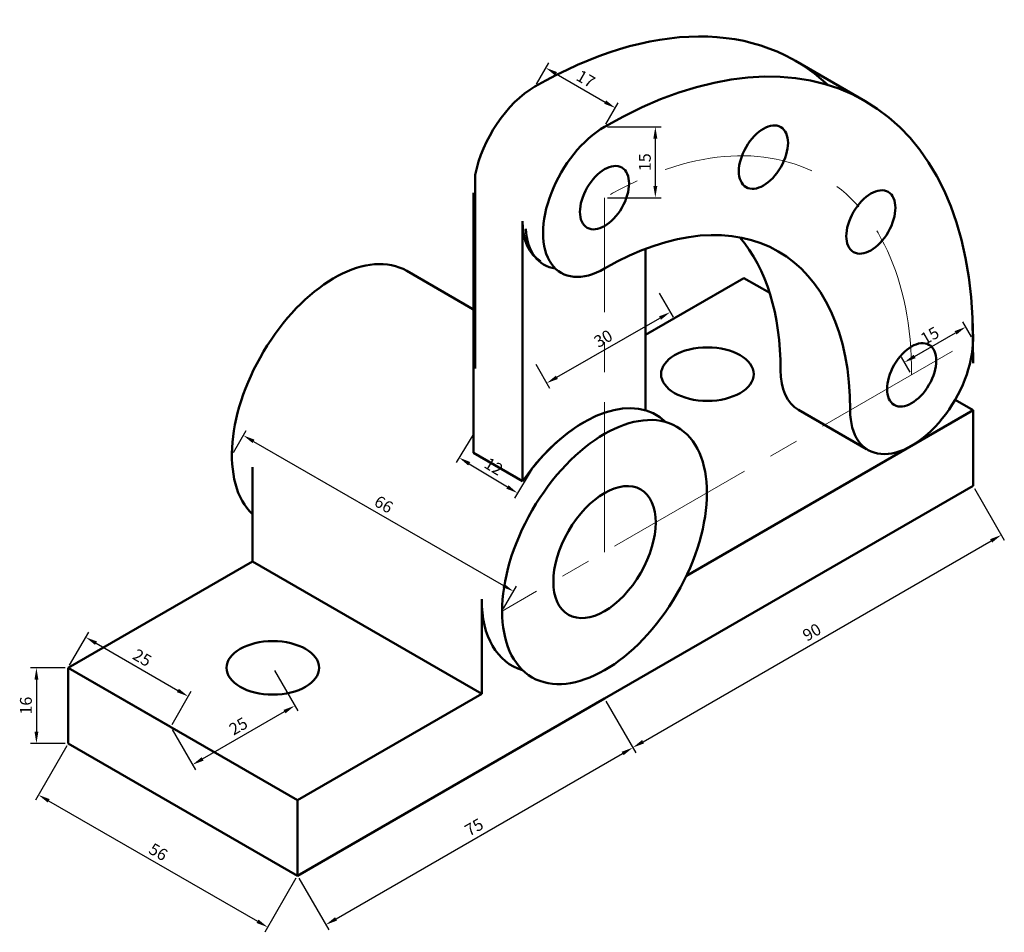
# Model space of a CAD drawing. Units: millimetres. Extents: x 2282 to 2491, y 1510 to 1704.
import ezdxf

# ---------------------------------------------------------------- set-up
doc = ezdxf.new("R2010")
doc.units = ezdxf.units.MM
doc.linetypes.add('CENTER', pattern=[50.8, 31.75, -6.35, 6.35, -6.35])
for name, color, linetype, lineweight in [('M-CNTR', 4, 'CENTER', 18), ('M-DIMS', 2, 'Continuous', 25), ('M-OUTL', 7, 'Continuous', 50)]:
    doc.layers.add(name, color=color, linetype=linetype, lineweight=lineweight)
doc.styles.get("Standard").update_dxf_attribs({"font": 'arial.ttf'})
doc.dimstyles.new('ISO-25', dxfattribs={"dimtxt": 2.5, "dimasz": 2.5, "dimexe": 1.25, "dimexo": 0.625, "dimtad": 1, "dimtxsty": 'Standard', "dimcen": 2.5, "dimadec": 0, "dimazin": 0, "dimtfac": 1, "dimtmove": 0, "dimatfit": 3, "dimfxl": 1, "dimarcsym": 0})

# ---------------------------------------------------------------- blocks, each defined once
blk = doc.blocks.new('*D1')
at = {"layer": 'Defpoints', "color": 0, "transparency": 16777216}
for p in [(2406.19, 1559.87), (2412.18, 1549.49), (2341.24, 1522.37)]:
    blk.add_point(p, dxfattribs=at)
at = {"layer": 'M-DIMS', "color": 0, "lineweight": -2, "transparency": 16777216}
for p, q in [((2406.5, 1559.33), (2412.81, 1548.41)), ((2349.4, 1513.24), (2410.02, 1548.24)), ((2341.55, 1521.83), (2347.86, 1510.91))]:
    blk.add_line(p, q, dxfattribs=at)
at = {"layer": 'M-DIMS', "color": 0, "transparency": 16777216}
for points in [[(2409.81, 1548.6), (2410.23, 1547.88), (2412.18, 1549.49)], [(2349.19, 1513.6), (2349.6, 1512.88), (2347.23, 1511.99)]]:
    blk.add_solid(points, dxfattribs=at)
at = {"layer": 'M-DIMS', "color": 0, "transparency": 16777216, "insert": (2378.76, 1532.38), "char_height": 2.5, "attachment_point": 5, "rotation": 30}
blk.add_mtext('75', dxfattribs=at)
blk = doc.blocks.new('*D2')
at = {"layer": 'Defpoints', "color": 0, "transparency": 16777216}
for p in [(2484.13, 1604.87), (2490.12, 1594.49), (2406.19, 1559.87)]:
    blk.add_point(p, dxfattribs=at)
at = {"layer": 'M-DIMS', "color": 0, "lineweight": -2, "transparency": 16777216}
for p, q in [((2484.45, 1604.33), (2490.75, 1593.41)), ((2414.35, 1550.74), (2487.96, 1593.24)), ((2406.5, 1559.33), (2412.81, 1548.41))]:
    blk.add_line(p, q, dxfattribs=at)
at = {"layer": 'M-DIMS', "color": 0, "transparency": 16777216}
for points in [[(2487.75, 1593.6), (2488.17, 1592.88), (2490.12, 1594.49)], [(2414.14, 1551.1), (2414.56, 1550.38), (2412.18, 1549.49)]]:
    blk.add_solid(points, dxfattribs=at)
at = {"layer": 'M-DIMS', "color": 0, "transparency": 16777216, "insert": (2450.2, 1573.64), "char_height": 2.5, "attachment_point": 5, "rotation": 30}
blk.add_mtext('90', dxfattribs=at)
blk = doc.blocks.new('*D3')
at = {"layer": 'Defpoints', "color": 0, "transparency": 16777216}
for p in [(2292.74, 1550.37), (2341.24, 1522.37), (2334.95, 1511.48)]:
    blk.add_point(p, dxfattribs=at)
at = {"layer": 'M-DIMS', "color": 0, "lineweight": -2, "transparency": 16777216}
for p, q in [((2292.43, 1549.83), (2285.83, 1538.4)), ((2288.62, 1538.23), (2332.79, 1512.73)), ((2340.93, 1521.83), (2334.33, 1510.4))]:
    blk.add_line(p, q, dxfattribs=at)
at = {"layer": 'M-DIMS', "color": 0, "transparency": 16777216}
for points in [[(2288.83, 1538.59), (2288.41, 1537.87), (2286.46, 1539.48)], [(2333, 1513.09), (2332.58, 1512.37), (2334.95, 1511.48)]]:
    blk.add_solid(points, dxfattribs=at)
at = {"layer": 'M-DIMS', "color": 0, "transparency": 16777216, "insert": (2311.65, 1527.13), "char_height": 2.5, "attachment_point": 5, "rotation": 330}
blk.add_mtext('56', dxfattribs=at)
blk = doc.blocks.new('*D4')
at = {"layer": 'Defpoints', "color": 0, "transparency": 16777216}
for p in [(2292.74, 1566.37), (2286.03, 1550.37), (2292.74, 1550.37)]:
    blk.add_point(p, dxfattribs=at)
at = {"layer": 'M-DIMS', "color": 0, "lineweight": -2, "transparency": 16777216}
for p, q in [((2292.12, 1566.37), (2284.78, 1566.37)), ((2286.03, 1563.87), (2286.03, 1552.87)), ((2292.12, 1550.37), (2284.78, 1550.37))]:
    blk.add_line(p, q, dxfattribs=at)
at = {"layer": 'M-DIMS', "color": 0, "transparency": 16777216}
for points in [[(2285.62, 1563.87), (2286.45, 1563.87), (2286.03, 1566.37)], [(2285.62, 1552.87), (2286.45, 1552.87), (2286.03, 1550.37)]]:
    blk.add_solid(points, dxfattribs=at)
at = {"layer": 'M-DIMS', "color": 0, "transparency": 16777216, "insert": (2284.13, 1558.37), "char_height": 2.5, "attachment_point": 5, "rotation": 90}
blk.add_mtext('16', dxfattribs=at)
blk = doc.blocks.new('*D5')
at = {"layer": 'Defpoints', "color": 0, "transparency": 16777216}
for p in [(2378.86, 1616.49), (2391.21, 1608.99), (2387.79, 1603.35)]:
    blk.add_point(p, dxfattribs=at)
at = {"layer": 'M-DIMS', "color": 0, "lineweight": -2, "transparency": 16777216}
for p, q in [((2378.53, 1615.96), (2374.78, 1609.79)), ((2377.57, 1609.56), (2385.65, 1604.65)), ((2390.89, 1608.45), (2387.14, 1602.28))]:
    blk.add_line(p, q, dxfattribs=at)
at = {"layer": 'M-DIMS', "color": 0, "transparency": 16777216}
for points in [[(2377.79, 1609.92), (2377.35, 1609.2), (2375.43, 1610.86)], [(2385.87, 1605.01), (2385.43, 1604.29), (2387.79, 1603.35)]]:
    blk.add_solid(points, dxfattribs=at)
at = {"layer": 'M-DIMS', "color": 0, "transparency": 16777216, "insert": (2382.59, 1608.71), "char_height": 2.5, "attachment_point": 5, "rotation": 328.7157}
blk.add_mtext('12', dxfattribs=at)
blk = doc.blocks.new('*D6')
at = {"layer": 'Defpoints', "color": 0, "transparency": 16777216}
for p in [(2417.45, 1646.22), (2420.08, 1641.64), (2391.32, 1631.19)]:
    blk.add_point(p, dxfattribs=at)
at = {"layer": 'M-DIMS', "color": 0, "lineweight": -2, "transparency": 16777216}
for p, q in [((2417.76, 1645.67), (2420.71, 1640.56)), ((2396.12, 1627.86), (2417.92, 1640.39)), ((2391.64, 1630.65), (2394.58, 1625.53))]:
    blk.add_line(p, q, dxfattribs=at)
at = {"layer": 'M-DIMS', "color": 0, "transparency": 16777216}
for points in [[(2417.71, 1640.75), (2418.12, 1640.03), (2420.08, 1641.64)], [(2395.92, 1628.22), (2396.33, 1627.5), (2393.96, 1626.62)]]:
    blk.add_solid(points, dxfattribs=at)
at = {"layer": 'M-DIMS', "color": 0, "transparency": 16777216, "insert": (2406.07, 1635.78), "char_height": 2.5, "attachment_point": 5, "rotation": 29.8992}
blk.add_mtext('30', dxfattribs=at)
blk = doc.blocks.new('*D7')
at = {"layer": 'Defpoints', "color": 0, "transparency": 16777216}
for p in [(2327.38, 1611.37), (2386.95, 1582.55), (2384.54, 1578.37)]:
    blk.add_point(p, dxfattribs=at)
at = {"layer": 'M-DIMS', "color": 0, "lineweight": -2, "transparency": 16777216}
for p, q in [((2327.7, 1611.91), (2330.42, 1616.63)), ((2331.96, 1614.3), (2384.79, 1583.8)), ((2384.85, 1578.91), (2387.58, 1583.63))]:
    blk.add_line(p, q, dxfattribs=at)
at = {"layer": 'M-DIMS', "color": 0, "transparency": 16777216}
for points in [[(2332.17, 1614.66), (2331.75, 1613.94), (2329.8, 1615.55)], [(2385, 1584.16), (2384.58, 1583.44), (2386.95, 1582.55)]]:
    blk.add_solid(points, dxfattribs=at)
at = {"layer": 'M-DIMS', "color": 0, "transparency": 16777216, "insert": (2359.33, 1600.69), "char_height": 2.5, "attachment_point": 5, "rotation": 330}
blk.add_mtext('66', dxfattribs=at)
blk = doc.blocks.new('*D8')
at = {"layer": 'Defpoints', "color": 0, "transparency": 16777216}
for p in [(2391.47, 1689.37), (2408.49, 1684.85), (2406.19, 1680.87)]:
    blk.add_point(p, dxfattribs=at)
at = {"layer": 'M-DIMS', "color": 0, "lineweight": -2, "transparency": 16777216}
for p, q in [((2391.78, 1689.91), (2394.39, 1694.43)), ((2395.93, 1692.1), (2406.32, 1686.1)), ((2406.5, 1681.41), (2409.11, 1685.93))]:
    blk.add_line(p, q, dxfattribs=at)
at = {"layer": 'M-DIMS', "color": 0, "transparency": 16777216}
for points in [[(2396.14, 1692.46), (2395.72, 1691.74), (2393.77, 1693.35)], [(2406.53, 1686.46), (2406.12, 1685.74), (2408.49, 1684.85)]]:
    blk.add_solid(points, dxfattribs=at)
at = {"layer": 'M-DIMS', "color": 0, "transparency": 16777216, "insert": (2402.07, 1690.73), "char_height": 2.5, "attachment_point": 5, "rotation": 330}
blk.add_mtext('17', dxfattribs=at)
blk = doc.blocks.new('*D9')
at = {"layer": 'Defpoints', "color": 0, "transparency": 16777216}
for p in [(2482.6, 1638.52), (2484.13, 1635.87), (2471.14, 1628.37)]:
    blk.add_point(p, dxfattribs=at)
at = {"layer": 'M-DIMS', "color": 0, "lineweight": -2, "transparency": 16777216}
for p, q in [((2483.82, 1636.41), (2481.98, 1639.6)), ((2471.78, 1632.27), (2480.44, 1637.27)), ((2470.83, 1628.91), (2468.99, 1632.1))]:
    blk.add_line(p, q, dxfattribs=at)
at = {"layer": 'M-DIMS', "color": 0, "transparency": 16777216}
for points in [[(2480.23, 1637.63), (2480.65, 1636.91), (2482.6, 1638.52)], [(2471.57, 1632.63), (2471.99, 1631.91), (2469.61, 1631.02)]]:
    blk.add_solid(points, dxfattribs=at)
at = {"layer": 'M-DIMS', "color": 0, "transparency": 16777216, "insert": (2475.16, 1636.41), "char_height": 2.5, "attachment_point": 5, "rotation": 30}
blk.add_mtext('15', dxfattribs=at)
blk = doc.blocks.new('*D10')
at = {"layer": 'Defpoints', "color": 0, "transparency": 16777216}
for p in [(2406.19, 1680.87), (2416.94, 1680.87), (2406.19, 1665.87)]:
    blk.add_point(p, dxfattribs=at)
at = {"layer": 'M-DIMS', "color": 0, "lineweight": -2, "transparency": 16777216}
for p, q in [((2406.82, 1680.87), (2418.19, 1680.87)), ((2416.94, 1668.37), (2416.94, 1678.37)), ((2406.82, 1665.87), (2418.19, 1665.87))]:
    blk.add_line(p, q, dxfattribs=at)
at = {"layer": 'M-DIMS', "color": 0, "transparency": 16777216}
for points in [[(2416.52, 1678.37), (2417.36, 1678.37), (2416.94, 1680.87)], [(2416.52, 1668.37), (2417.36, 1668.37), (2416.94, 1665.87)]]:
    blk.add_solid(points, dxfattribs=at)
at = {"layer": 'M-DIMS', "color": 0, "transparency": 16777216, "insert": (2415.04, 1673.37), "char_height": 2.5, "attachment_point": 5, "rotation": 90}
blk.add_mtext('15', dxfattribs=at)
blk = doc.blocks.new('*D11')
at = {"layer": 'Defpoints', "color": 0, "transparency": 16777216}
for p in [(2336.04, 1566.37), (2340.67, 1558.35), (2314.39, 1553.87)]:
    blk.add_point(p, dxfattribs=at)
at = {"layer": 'M-DIMS', "color": 0, "lineweight": -2, "transparency": 16777216}
for p, q in [((2336.36, 1565.83), (2341.3, 1557.27)), ((2321.19, 1547.1), (2338.51, 1557.1)), ((2314.71, 1553.33), (2319.65, 1544.77))]:
    blk.add_line(p, q, dxfattribs=at)
at = {"layer": 'M-DIMS', "color": 0, "transparency": 16777216}
for points in [[(2338.3, 1557.46), (2338.71, 1556.74), (2340.67, 1558.35)], [(2320.98, 1547.46), (2321.39, 1546.74), (2319.02, 1545.85)]]:
    blk.add_solid(points, dxfattribs=at)
at = {"layer": 'M-DIMS', "color": 0, "transparency": 16777216, "insert": (2328.9, 1553.75), "char_height": 2.5, "attachment_point": 5, "rotation": 30}
blk.add_mtext('25', dxfattribs=at)
blk = doc.blocks.new('*D12')
at = {"layer": 'Defpoints', "color": 0, "transparency": 16777216}
for p in [(2292.74, 1566.37), (2318.12, 1560.33), (2314.39, 1553.87)]:
    blk.add_point(p, dxfattribs=at)
at = {"layer": 'M-DIMS', "color": 0, "lineweight": -2, "transparency": 16777216}
for p, q in [((2293.05, 1566.91), (2297.1, 1573.91)), ((2298.64, 1571.58), (2315.96, 1561.58)), ((2314.71, 1554.41), (2318.75, 1561.41))]:
    blk.add_line(p, q, dxfattribs=at)
at = {"layer": 'M-DIMS', "color": 0, "transparency": 16777216}
for points in [[(2298.85, 1571.94), (2298.43, 1571.22), (2296.47, 1572.83)], [(2316.17, 1561.94), (2315.75, 1561.22), (2318.12, 1560.33)]]:
    blk.add_solid(points, dxfattribs=at)
at = {"layer": 'M-DIMS', "color": 0, "transparency": 16777216, "insert": (2308.25, 1568.23), "char_height": 2.5, "attachment_point": 5, "rotation": 330}
blk.add_mtext('25', dxfattribs=at)

msp = doc.modelspace()

# ---------------------------------------------------------------- linework, layer by layer
at = {"layer": 'M-CNTR'}
for p, q in [((2406.191, 1590.869), (2406.191, 1665.869)), ((2479.803, 1633.369), (2384.541, 1578.369))]:
    msp.add_line(p, q, dxfattribs=at)
msp.add_ellipse((2406.191, 1590.869), major_axis=(-45.928, -79.55), ratio=0.5773503, start_param=8.6393798, end_param=10.2101761, dxfattribs=at)
at = {"layer": 'M-OUTL'}
for p, q in [((2446.582, 1694.828), (2461.305, 1686.328)), ((2378.857, 1670.681), (2378.857, 1629.727)), ((2378.478, 1611.869), (2378.478, 1666.869)), ((2388.871, 1605.869), (2388.871, 1660.869)), ((2414.851, 1620.869), (2414.851, 1655.03)), ((2364.343, 1650.386), (2378.857, 1642.006)), ((2414.851, 1636.869), (2435.636, 1648.869)), ((2441.129, 1645.697), (2435.636, 1648.869)), ((2484.134, 1630.869), (2484.049, 1640)), ((2484.134, 1620.869), (2480.329, 1623.066)), ((2423.512, 1585.869), (2484.134, 1620.869)), ((2461.6, 1612.682), (2447.24, 1620.956)), ((2484.134, 1604.869), (2484.134, 1620.869)), ((2388.871, 1605.869), (2378.478, 1611.869)), ((2331.713, 1608.869), (2331.713, 1588.869)), ((2406.191, 1559.869), (2484.134, 1604.869)), ((2292.742, 1566.369), (2331.713, 1588.869)), ((2380.21, 1560.869), (2331.713, 1588.869)), ((2380.21, 1580.869), (2380.21, 1560.869)), ((2292.742, 1550.369), (2292.742, 1566.369)), ((2292.742, 1566.369), (2341.239, 1538.369)), ((2292.742, 1566.369), (2314.393, 1553.869)), ((2341.239, 1538.369), (2380.21, 1560.869)), ((2341.239, 1522.369), (2406.191, 1559.869)), ((2341.239, 1522.369), (2292.742, 1550.369)), ((2341.239, 1522.369), (2341.239, 1538.369))]:
    msp.add_line(p, q, dxfattribs=at)
for centre, major_axis, start_param, end_param in [((2391.469, 1599.369), (-55.114, -95.459), 3.0076277, 3.9269908), ((2406.191, 1590.869), (-55.114, -95.459), 2.3561945, 3.9269908), ((2391.469, 1674.369), (-9.186, -15.91), 3.9269908, 5.2558829), ((2391.469, 1674.369), (-9.186, -15.91), 3.9269908, 5.2558829), ((2406.191, 1665.869), (-9.186, -15.91), 3.9269908, 7.0685835), ((2401.861, 1668.369), (-9.186, -15.91), 5.4977871, 6.2831853), ((2406.191, 1590.869), (-36.742, -63.64), 8.6393798, 10.2101761), ((2402.53, 1667.61), (-9.186, -15.91), 5.5562934, 6.5211264), ((2391.469, 1599.369), (-36.742, -63.64), 8.6393798, 9.223066), ((2349.034, 1623.869), (-15.309, -26.517), 3.1415927, 6.1412883), ((2471.143, 1628.369), (-9.186, -15.91), 5.4977871, 8.6393798), ((2456.421, 1636.869), (-9.186, -15.91), 5.4977871, 6.2836899), ((2401.861, 1593.369), (-15.309, -26.517), 2.9996956, 4.4412878), ((2401.861, 1593.369), (15.309, 26.517), 0.7853982, 1.4288993), ((2401.861, 1593.369), (-15.309, -26.517), 5.4977871, 6.4250824)]:
    msp.add_ellipse(centre, major_axis=major_axis, ratio=0.5773503, start_param=start_param, end_param=end_param, dxfattribs=at)
for centre, major_axis in [((2439.804, 1674.452), (-3.674, -6.364)), ((2406.191, 1665.869), (-3.674, -6.364)), ((2462.527, 1660.722), (-3.674, -6.364)), ((2471.143, 1628.369), (-3.674, -6.364)), ((2427.951, 1628.523), (-9.798, 0)), ((2406.191, 1590.869), (-15.309, -26.517)), ((2406.191, 1590.869), (-7.655, -13.258)), ((2336.043, 1566.369), (-9.798, 0))]:
    msp.add_ellipse(centre, major_axis=major_axis, ratio=0.5773503, dxfattribs=at)

# ---------------------------------------------------------------- dimensions: what is measured, and where the dimension line sits
at = {"layer": 'M-DIMS'}
for p1, p2, distance, picture, middle in [((2391.469, 1689.369), (2406.191, 1680.869), 4.595, '*D8', (2402.068, 1690.727)), ((2406.191, 1665.869), (2406.191, 1680.869), -10.75, '*D10', (2415.04, 1673.369)), ((2471.143, 1628.369), (2484.134, 1635.869), 3.058, '*D9', (2475.159, 1636.414)), ((2327.383, 1611.369), (2384.541, 1578.369), 4.825, '*D7', (2359.325, 1600.694)), ((2406.191, 1559.869), (2484.134, 1604.869), -11.982, '*D2', (2450.203, 1573.639)), ((2292.742, 1566.369), (2314.393, 1553.869), 7.46, '*D12', (2308.248, 1568.227)), ((2292.742, 1566.369), (2292.742, 1550.369), -6.708, '*D4', (2284.133, 1558.369)), ((2314.393, 1553.869), (2336.043, 1566.369), -9.256, '*D11', (2328.895, 1553.75)), ((2341.239, 1522.369), (2406.191, 1559.869), -11.982, '*D1', (2378.758, 1532.385)), ((2292.742, 1550.369), (2341.239, 1522.369), -12.574, '*D3', (2311.655, 1527.127))]:
    dim = msp.add_aligned_dim(p1=p1, p2=p2, distance=distance, dimstyle='ISO-25', override={"dimclrd": 0, "dimclre": 0, "dimclrt": 0}, dxfattribs=at)
    dim.commit()
    dim.dimension.update_dxf_attribs({"geometry": picture, "text_midpoint": middle})
for p1, p2, distance, text, picture, middle in [((2391.324, 1631.192), (2417.452, 1646.216), -5.28, '30', '*D6', (2406.072, 1635.776)), ((2378.857, 1616.493), (2391.211, 1608.986), -6.592, '12', '*D5', (2382.587, 1608.712))]:
    dim = msp.add_aligned_dim(p1=p1, p2=p2, distance=distance, text=text, dimstyle='ISO-25', override={"dimclrd": 0, "dimclre": 0, "dimclrt": 0}, dxfattribs=at)
    dim.commit()
    dim.dimension.update_dxf_attribs({"geometry": picture, "text_midpoint": middle})

doc.saveas('drawing.dxf')
